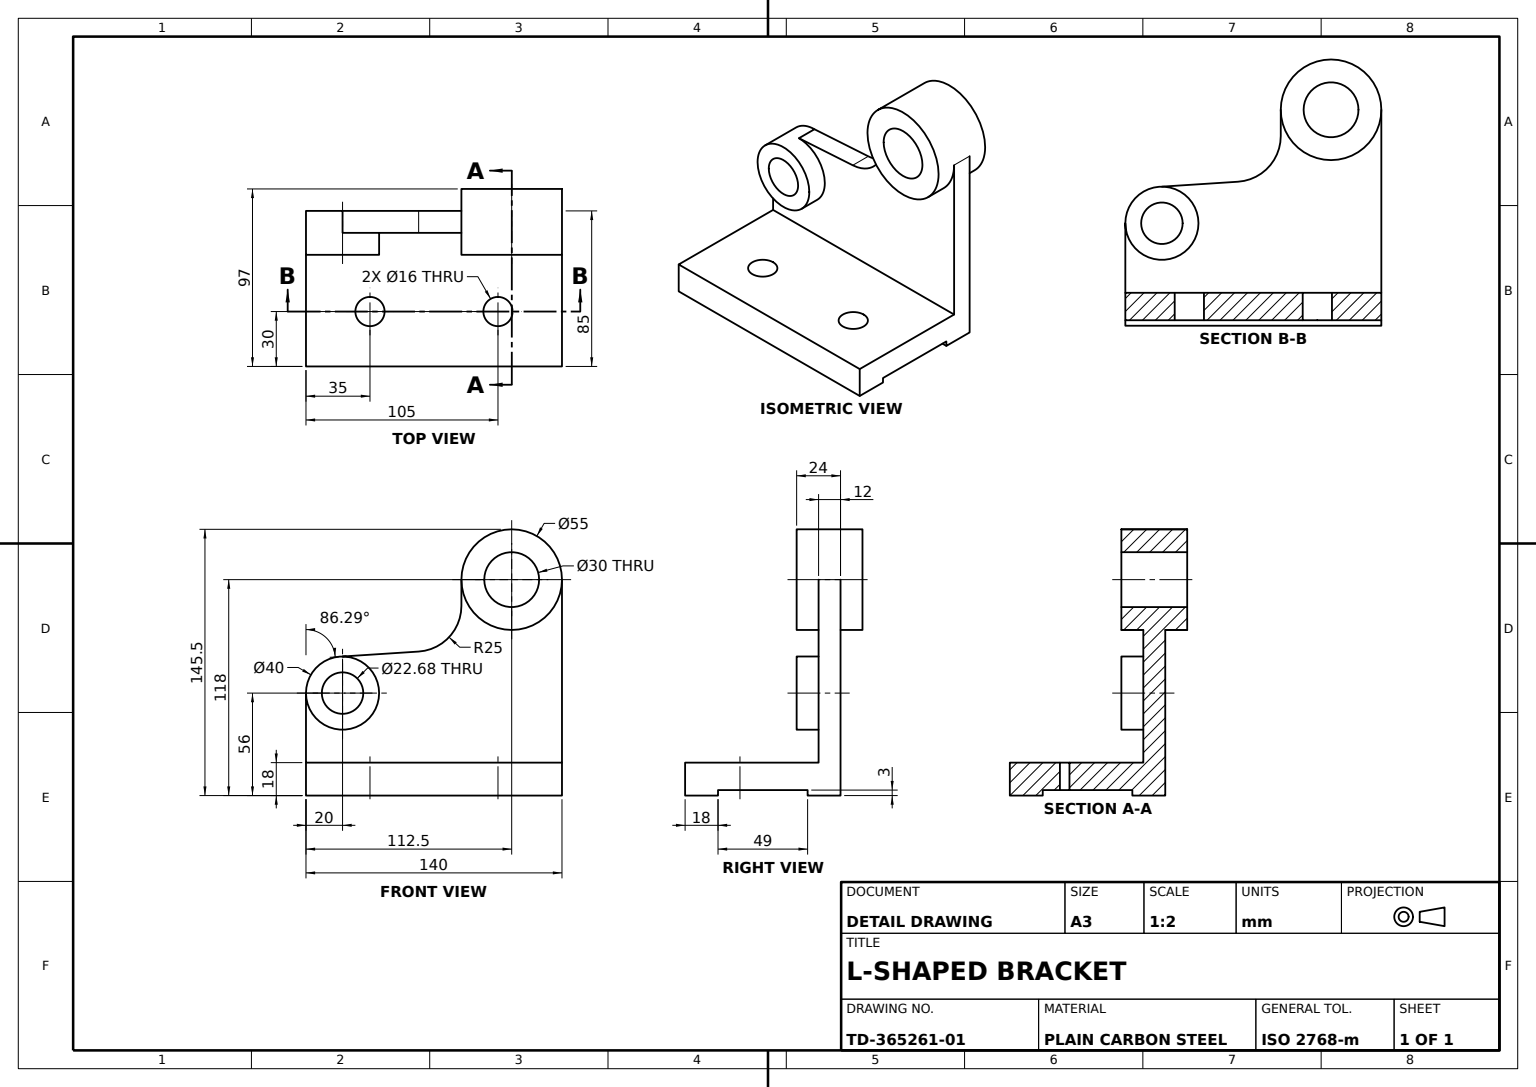
from build123d import *

# Parameters (mm, degrees)
BASE_PLATE_SKETCH_W              = 140
BASE_PLATE_SKETCH_H              = 85
BASE_PLATE_85X140X18_DEPTH       = 18
UNDERSIDE_GROOVE_SKETCH_W        = 49
UNDERSIDE_GROOVE_SKETCH_H        = 3
UNDERSIDE_GROOVE_DEPTH           = 140
UPRIGHT_WALL_SKETCH_W            = 140
UPRIGHT_WALL_SKETCH_H            = 12
UPRIGHT_WALL_DEPTH               = 100
SMALL_LUG_40_SKETCH_R            = 20
SMALL_LUG_40_DEPTH               = 12
LARGE_LUG_55_SKETCH_R            = 27.5
LARGE_LUG_55_DEPTH               = 24
LARGE_START                      = 12
LARGE_LUG_EXTENSION_SKETCH_R     = 27.5
LARGE_LUG_EXTENSION_DEPTH        = 12
LUG_START                        = -12
LUG_RELIEF_CUT_DEPTH             = 12
LARGE_LUG_BORE_30_SKETCH_R       = 15
LARGE_LUG_BORE_30_DEPTH          = 36
SMALL_LUG_BORE_SKETCH_R          = 11.34199473
SMALL_LUG_BORE_DEPTH             = 36
BASE_MOUNTING_HOLE_1_16_SKETCH_R = 8
BASE_MOUNTING_HOLE_1_16_DEPTH    = 15
BASE_MOUNTING_HOLE_2_16_SKETCH_R = 8
BASE_MOUNTING_HOLE_2_16_DEPTH    = 15


with BuildPart() as part:
    # Base Plate Sketch → Base Plate 85x140x18 (new body)
    with BuildSketch(Plane(origin=(0, 0, 0), x_dir=(1, 0, 0), z_dir=(0, 1, 0))):
        Rectangle(BASE_PLATE_SKETCH_W, BASE_PLATE_SKETCH_H)
    extrude(amount=BASE_PLATE_85X140X18_DEPTH)

    # Underside Groove Sketch → Underside Groove (cut)
    with BuildSketch(Plane(origin=(70, 0, 0), x_dir=(0, 0, -1), z_dir=(1, 0, 0))):
        with Locations((0, 1.5)):
            Rectangle(UNDERSIDE_GROOVE_SKETCH_W, UNDERSIDE_GROOVE_SKETCH_H)
    extrude(amount=-UNDERSIDE_GROOVE_DEPTH, mode=Mode.SUBTRACT)

    # Upright Wall Sketch → Upright Wall (add)
    with BuildSketch(Plane(origin=(0, 18, 0), x_dir=(1, 0, 0), z_dir=(0, 1, 0))):
        with Locations((0, 36.5)):
            Rectangle(UPRIGHT_WALL_SKETCH_W, UPRIGHT_WALL_SKETCH_H)
    extrude(amount=UPRIGHT_WALL_DEPTH)

    # Small Lug Ø40 Sketch → Small Lug Ø40 (add)
    with BuildSketch(Plane.XY.offset(-30.5)):
        with Locations(Location((-50, 56, 0), (0, 0, 180))):
            Circle(SMALL_LUG_40_SKETCH_R)
    extrude(amount=SMALL_LUG_40_DEPTH)

    # Large Lug Ø55 Sketch → Large Lug Ø55 (add)
    with BuildSketch(Plane.XY.offset(-30.5)):
        with Locations((42.5, 118)):
            Circle(LARGE_LUG_55_SKETCH_R)
    extrude(amount=-LARGE_LUG_55_DEPTH)

    # Large Lug Extension Sketch → Large Lug Extension (add)
    with BuildSketch(Plane.XY.offset(-30.5).offset(LARGE_START)):
        with Locations((42.5, 118)):
            Circle(LARGE_LUG_EXTENSION_SKETCH_R)
    extrude(amount=-LARGE_LUG_EXTENSION_DEPTH)

    # Lug Relief Cut Sketch → Lug Relief Cut (cut)
    with BuildSketch(Plane.XY.offset(-30.5).offset(LUG_START)):
        with BuildLine():
            Line((15, 118), (15, 103.64309486))
            ThreePointArc((15, 103.64309486), (8.240000897, 86.546242306), (-8.384189381, 78.695366386))
            Line((-8.384189381, 78.695366386), (-50, 76))
            ThreePointArc((-50, 76), (-64.142135624, 70.142135624), (-70, 56))
            Line((-70, 56), (-70, 118))
            Line((-70, 118), (15, 118))
        make_face()
    extrude(amount=LUG_RELIEF_CUT_DEPTH, mode=Mode.SUBTRACT)

    # Large Lug Bore Ø30 Sketch → Large Lug Bore Ø30 (cut)
    with BuildSketch(Plane.XY.offset(-18.5)):
        with Locations((42.5, 118)):
            Circle(LARGE_LUG_BORE_30_SKETCH_R)
    extrude(amount=-LARGE_LUG_BORE_30_DEPTH, mode=Mode.SUBTRACT)

    # Small Lug Bore Sketch → Small Lug Bore (cut)
    with BuildSketch(Plane.XY.offset(-18.5)):
        with Locations((-50, 56)):
            Circle(SMALL_LUG_BORE_SKETCH_R)
    extrude(amount=-SMALL_LUG_BORE_DEPTH, mode=Mode.SUBTRACT)

    # Base Mounting Hole 1 Ø16 Sketch → Base Mounting Hole 1 Ø16 (cut)
    with BuildSketch(Plane(origin=(0, 18, 0), x_dir=(1, 0, 0), z_dir=(0, 1, 0))):
        with Locations(Location((-35, -12.5, 0), (0, 0, 270))):
            Circle(BASE_MOUNTING_HOLE_1_16_SKETCH_R)
    extrude(amount=-BASE_MOUNTING_HOLE_1_16_DEPTH, mode=Mode.SUBTRACT)

    # Base Mounting Hole 2 Ø16 Sketch → Base Mounting Hole 2 Ø16 (cut)
    with BuildSketch(Plane(origin=(0, 18, 0), x_dir=(1, 0, 0), z_dir=(0, 1, 0))):
        with Locations(Location((35, -12.5, 0), (0, 0, 270))):
            Circle(BASE_MOUNTING_HOLE_2_16_SKETCH_R)
    extrude(amount=-BASE_MOUNTING_HOLE_2_16_DEPTH, mode=Mode.SUBTRACT)


solid = part.part
